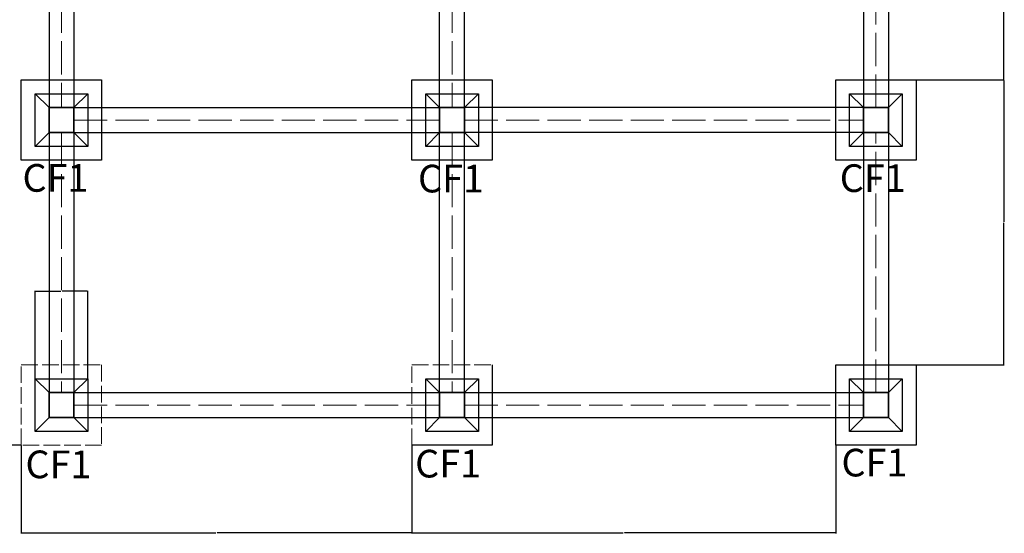
# Model space of a CAD drawing. Units: inches. Extents: x -154 to 668, y -797 to 97.
# Tile 2 of 4: x 313 to 668, y -552 to -367. Entities that reach past the tile are written whole.
import ezdxf

# ---------------------------------------------------------------- set-up
doc = ezdxf.new("R2010")
doc.units = ezdxf.units.IN
doc.header["$MEASUREMENT"] = 0
doc.linetypes.add('ACAD_ISO02W100', pattern=[15, 12, -3])
for name, color, linetype, lineweight in [('A-ANNO-DIMS', 2, 'Continuous', 18), ('S-ANNO-IDEN', 7, 'Continuous', 18), ('S-BEAM', 152, 'Continuous', 25), ('S-BEAM-CNTR', 2, 'ACAD_ISO02W100', 13), ('S-COLS', 2, 'Continuous', 35), ('S-FNDN', 2, 'Continuous', 30), ('S-FNDN-BASE-HIDN', 7, 'ACAD_ISO02W100', 18)]:
    doc.layers.add(name, color=color, linetype=linetype, lineweight=lineweight)
doc.styles.get("Standard").update_dxf_attribs({"font": 'arial.ttf'})
doc.dimstyles.get("Standard").update_dxf_attribs({"dimtxt": 0.18, "dimasz": 0.18, "dimexe": 0.18, "dimexo": 0.0625, "dimgap": 0.09, "dimtad": 0, "dimtih": 1, "dimtoh": 1, "dimdec": 1, "dimzin": 0, "dimdsep": 46, "dimlunit": 4, "dimtxsty": 'Standard', "dimcen": 0.09, "dimadec": 0, "dimazin": 0, "dimtfac": 1, "dimtdec": 1, "dimtofl": 0, "dimtmove": 0, "dimatfit": 3, "dimfxl": 1, "dimtolj": 1, "dimtzin": 0, "dimarcsym": 0})

# ---------------------------------------------------------------- blocks, each defined once
blk = doc.blocks.new('COLUMN-9X9')
for p, q in [((-4.5, 4.5), (4.5, 4.5)), ((-4.5, -4.5), (-4.5, 4.5)), ((4.5, 4.5), (4.5, -4.5)), ((4.5, -4.5), (-4.5, -4.5))]:
    blk.add_line(p, q)
blk = doc.blocks.new('CF1-ISOLATED-FOOTING')
for p, q in [((-14.5, 14.5), (14.5, 14.5)), ((-14.5, -14.5), (-14.5, 14.5)), ((14.5, 14.5), (14.5, -14.5)), ((-9.5, 9.5), (9.5, 9.5)), ((-9.5, -9.5), (-9.5, 9.5)), ((-9.5, 9.5), (-4.5, 4.5)), ((4.5, 4.5), (9.5, 9.5)), ((9.5, 9.5), (9.5, -9.5)), ((-9.5, -9.5), (-4.5, -4.5)), ((4.5, -4.5), (9.5, -9.5)), ((9.5, -9.5), (-9.5, -9.5)), ((14.5, -14.5), (-14.5, -14.5))]:
    blk.add_line(p, q)
blk = doc.blocks.new('*D51')
at = {"layer": 'A-ANNO-DIMS', "color": 0, "lineweight": -2, "transparency": 16777216}
for p, q in [((313.34, 65.33), (281.57, 65.33)), ((281.75, 65.15), (281.75, -227.49)), ((281.75, -520.49), (281.75, -227.85)), ((313.34, -520.67), (281.57, -520.67))]:
    blk.add_line(p, q, dxfattribs=at)
at = {"layer": 'A-ANNO-DIMS', "color": 0, "transparency": 16777216}
for points in [[(281.72, 65.15), (281.78, 65.15), (281.75, 65.33)], [(281.72, -520.49), (281.78, -520.49), (281.75, -520.67)]]:
    blk.add_solid(points, dxfattribs=at)
at = {"layer": 'Defpoints', "color": 0, "transparency": 16777216}
for p in [(281.75, 65.33), (313.4, 65.33), (313.4, -520.67)]:
    blk.add_point(p, dxfattribs=at)
at = {"layer": 'A-ANNO-DIMS', "color": 0, "transparency": 16777216, "insert": (281.75, -227.67), "char_height": 0.18, "attachment_point": 5}
blk.add_mtext('\\A1;586', dxfattribs=at)
blk = doc.blocks.new('*D52')
at = {"layer": 'A-ANNO-DIMS', "color": 0, "lineweight": -2, "transparency": 16777216}
for p, q in [((313.4, -520.73), (313.4, -552.5)), ((454.4, -520.73), (454.4, -552.5)), ((313.58, -552.32), (383.64, -552.32)), ((454.22, -552.32), (384.16, -552.32))]:
    blk.add_line(p, q, dxfattribs=at)
at = {"layer": 'A-ANNO-DIMS', "color": 0, "transparency": 16777216}
for points in [[(313.58, -552.29), (313.58, -552.35), (313.4, -552.32)], [(454.22, -552.29), (454.22, -552.35), (454.4, -552.32)]]:
    blk.add_solid(points, dxfattribs=at)
at = {"layer": 'Defpoints', "color": 0, "transparency": 16777216}
for p in [(313.4, -520.67), (454.4, -520.67), (454.4, -552.32)]:
    blk.add_point(p, dxfattribs=at)
at = {"layer": 'A-ANNO-DIMS', "color": 0, "transparency": 16777216, "insert": (383.9, -552.32), "char_height": 0.18, "attachment_point": 5}
blk.add_mtext('\\A1;141', dxfattribs=at)
blk = doc.blocks.new('*D53')
at = {"layer": 'A-ANNO-DIMS', "color": 0, "lineweight": -2, "transparency": 16777216}
for p, q in [((454.4, -520.73), (454.4, -552.5)), ((607.4, -520.73), (607.4, -552.5)), ((454.58, -552.32), (530.62, -552.32)), ((607.22, -552.32), (531.18, -552.32))]:
    blk.add_line(p, q, dxfattribs=at)
at = {"layer": 'A-ANNO-DIMS', "color": 0, "transparency": 16777216}
for points in [[(454.58, -552.29), (454.58, -552.35), (454.4, -552.32)], [(607.22, -552.29), (607.22, -552.35), (607.4, -552.32)]]:
    blk.add_solid(points, dxfattribs=at)
at = {"layer": 'Defpoints', "color": 0, "transparency": 16777216}
for p in [(454.4, -520.67), (607.4, -520.67), (607.4, -552.32)]:
    blk.add_point(p, dxfattribs=at)
at = {"layer": 'A-ANNO-DIMS', "color": 0, "transparency": 16777216, "insert": (530.9, -552.32), "char_height": 0.18, "attachment_point": 5}
blk.add_mtext('\\A1;153', dxfattribs=at)
blk = doc.blocks.new('*D59')
at = {"layer": 'A-ANNO-DIMS', "color": 0, "lineweight": -2, "transparency": 16777216}
for p, q in [((636.46, -235.67), (668.23, -235.67)), ((668.05, -235.85), (668.05, -311.99)), ((668.05, -388.49), (668.05, -312.35)), ((636.46, -388.67), (668.23, -388.67))]:
    blk.add_line(p, q, dxfattribs=at)
at = {"layer": 'A-ANNO-DIMS', "color": 0, "transparency": 16777216}
for points in [[(668.02, -235.85), (668.08, -235.85), (668.05, -235.67)], [(668.02, -388.49), (668.08, -388.49), (668.05, -388.67)]]:
    blk.add_solid(points, dxfattribs=at)
at = {"layer": 'Defpoints', "color": 0, "transparency": 16777216}
for p in [(636.4, -235.67), (668.05, -235.67), (636.4, -388.67)]:
    blk.add_point(p, dxfattribs=at)
at = {"layer": 'A-ANNO-DIMS', "color": 0, "transparency": 16777216, "insert": (668.05, -312.17), "char_height": 0.18, "attachment_point": 5}
blk.add_mtext('\\A1;153', dxfattribs=at)
blk = doc.blocks.new('*D60')
at = {"layer": 'A-ANNO-DIMS', "color": 0, "lineweight": -2, "transparency": 16777216}
for p, q in [((636.46, -388.67), (668.23, -388.67)), ((668.05, -388.85), (668.05, -439.99)), ((668.05, -491.49), (668.05, -440.35)), ((636.46, -491.67), (668.23, -491.67))]:
    blk.add_line(p, q, dxfattribs=at)
at = {"layer": 'A-ANNO-DIMS', "color": 0, "transparency": 16777216}
for points in [[(668.02, -388.85), (668.08, -388.85), (668.05, -388.67)], [(668.02, -491.49), (668.08, -491.49), (668.05, -491.67)]]:
    blk.add_solid(points, dxfattribs=at)
at = {"layer": 'Defpoints', "color": 0, "transparency": 16777216}
for p in [(636.4, -388.67), (668.05, -388.67), (636.4, -491.67)]:
    blk.add_point(p, dxfattribs=at)
at = {"layer": 'A-ANNO-DIMS', "color": 0, "transparency": 16777216, "insert": (668.05, -440.17), "char_height": 0.18, "attachment_point": 5}
blk.add_mtext('\\A1;103', dxfattribs=at)
blk = doc.blocks.new('*D61')
at = {"layer": 'A-ANNO-DIMS', "color": 0, "lineweight": -2, "transparency": 16777216}
for p, q in [((318.4, -496.6), (318.4, -464.84)), ((318.58, -465.02), (327.69, -465.02)), ((337.22, -465.02), (328.11, -465.02)), ((337.4, -496.6), (337.4, -464.84))]:
    blk.add_line(p, q, dxfattribs=at)
at = {"layer": 'A-ANNO-DIMS', "color": 0, "transparency": 16777216}
for points in [[(318.58, -464.99), (318.58, -465.05), (318.4, -465.02)], [(337.22, -464.99), (337.22, -465.05), (337.4, -465.02)]]:
    blk.add_solid(points, dxfattribs=at)
at = {"layer": 'Defpoints', "color": 0, "transparency": 16777216}
for p in [(337.4, -465.02), (318.4, -496.67), (337.4, -496.67)]:
    blk.add_point(p, dxfattribs=at)
at = {"layer": 'A-ANNO-DIMS', "color": 0, "transparency": 16777216, "insert": (327.9, -465.02), "char_height": 0.18, "attachment_point": 5}
blk.add_mtext('\\A1;19', dxfattribs=at)

msp = doc.modelspace()

# ---------------------------------------------------------------- linework, layer by layer
at = {"layer": 'S-BEAM'}
for p, q in [((323.3997, -254.6672), (323.3997, -407.6672)), ((332.3997, -254.6672), (332.3997, -398.6672)), ((464.3997, -398.6672), (464.3997, -254.6672)), ((473.3997, -398.6672), (473.3997, -254.6672)), ((617.3997, -254.6672), (617.3997, -398.6672)), ((626.3997, -254.6672), (626.3997, -510.6672)), ((332.3997, -398.6672), (464.3997, -398.6672)), ((617.3997, -398.6672), (473.3997, -398.6672)), ((323.3997, -407.6672), (464.3997, -407.6672)), ((323.3997, -407.6672), (323.3997, -510.6672)), ((332.3997, -407.6672), (332.3997, -501.6672)), ((617.3997, -407.6672), (464.3997, -407.6672)), ((464.3997, -501.6672), (464.3997, -407.6672)), ((473.3997, -501.6672), (473.3997, -407.6672)), ((617.3997, -407.6672), (617.3997, -501.6672)), ((332.3997, -501.6672), (464.3997, -501.6672)), ((464.3997, -501.6672), (617.3997, -501.6672)), ((464.3997, -501.6672), (464.3997, -510.6672)), ((323.3997, -510.6672), (626.3997, -510.6672))]:
    msp.add_line(p, q, dxfattribs=at)
at = {"layer": 'S-BEAM-CNTR'}
for p, q in [((327.8997, -254.6672), (327.8997, -398.6672)), ((468.8997, -254.6672), (468.8997, -398.6672)), ((621.8997, -398.6672), (621.8997, -254.6672)), ((332.3997, -403.1672), (464.3997, -403.1672)), ((473.3997, -403.1672), (617.3997, -403.1672)), ((327.8997, -407.6672), (327.8997, -501.6672)), ((468.8997, -407.6672), (468.8997, -501.6672)), ((621.8997, -501.6672), (621.8997, -407.6672)), ((332.3997, -506.1672), (464.3997, -506.1672)), ((473.3997, -506.1672), (617.3997, -506.1672))]:
    msp.add_line(p, q, dxfattribs=at)
at = {"layer": 'S-COLS'}
msp.add_line((617.3997, -407.6672), (617.3997, -398.6672), dxfattribs=at)
at = {"layer": 'S-FNDN'}
for p, q in [((483.3997, -491.6672), (483.3997, -520.6672)), ((318.3997, -515.6672), (318.3997, -496.6672)), ((318.3997, -496.6672), (337.3997, -496.6672)), ((318.3997, -496.6672), (323.3997, -501.6672)), ((332.3997, -501.6672), (337.3997, -496.6672)), ((337.3997, -496.6672), (337.3997, -515.6672)), ((459.3997, -515.6672), (459.3997, -496.6672)), ((459.3997, -496.6672), (478.3997, -496.6672)), ((459.3997, -496.6672), (464.3997, -501.6672)), ((473.3997, -501.6672), (478.3997, -496.6672)), ((478.3997, -496.6672), (478.3997, -515.6672)), ((318.3997, -515.6672), (323.3997, -510.6672)), ((332.3997, -510.6672), (337.3997, -515.6672)), ((459.3997, -515.6672), (464.3997, -510.6672)), ((473.3997, -510.6672), (478.3997, -515.6672)), ((337.3997, -515.6672), (318.3997, -515.6672)), ((478.3997, -515.6672), (459.3997, -515.6672)), ((483.3997, -520.6672), (454.3997, -520.6672))]:
    msp.add_line(p, q, dxfattribs=at)
at = {"layer": 'S-FNDN-BASE-HIDN', "ltscale": 0.5}
for p, q in [((313.3997, -520.6672), (313.3997, -491.6672)), ((313.3997, -491.6672), (342.3997, -491.6672)), ((342.3997, -491.6672), (342.3997, -520.6672)), ((454.3997, -520.6672), (454.3997, -491.6672)), ((454.3997, -491.6672), (483.3997, -491.6672)), ((342.3997, -520.6672), (313.3997, -520.6672))]:
    msp.add_line(p, q, dxfattribs=at)

# ---------------------------------------------------------------- block references
at = {"layer": 'S-COLS'}
for p, rotation in [((327.8995, -403.1669), 89.99999999999893), ((468.8995, -403.1669), 90.00000000000036), ((621.8995, -403.1669), 89.99999999999964), ((327.8995, -506.1669), 89.99999999999893), ((468.8995, -506.1669), 90.00000000000074), ((621.8995, -506.1669), 89.99999999999964)]:
    msp.add_blockref('COLUMN-9X9', p, dxfattribs=dict(at, rotation=rotation))
at = {"layer": 'S-FNDN'}
msp.add_blockref('CF1-ISOLATED-FOOTING', (327.9, -403.167), dxfattribs=at)
for p, rotation in [((468.8994, -403.1674), 180), ((621.8994, -403.1674), 180), ((621.8995, -506.1669), 90.00000000000094)]:
    msp.add_blockref('CF1-ISOLATED-FOOTING', p, dxfattribs=dict(at, rotation=rotation))

# ---------------------------------------------------------------- texts
at = {"layer": 'S-ANNO-IDEN'}
for p in [(313.8292, -429.0678), (456.6003, -429.324), (608.8568, -429.1612), (314.9035, -532.5782), (455.5679, -532.3219), (609.4674, -531.9476)]:
    msp.add_text('CF1', height=10, dxfattribs=at).set_placement(p)

# ---------------------------------------------------------------- dimensions: what is measured, and where the dimension line sits
at = {"layer": 'A-ANNO-DIMS'}
for base, p1, p2, picture, middle in [((281.7497, 65.3328), (313.3997, -520.6672), (313.3997, 65.3328), '*D51', (281.7497, -227.6672)), ((668.0497, -235.6672), (636.3997, -388.6672), (636.3997, -235.6672), '*D59', (668.0497, -312.1672)), ((668.0497, -388.6672), (636.3997, -491.6672), (636.3997, -388.6672), '*D60', (668.0497, -440.1672))]:
    dim = msp.add_linear_dim(base=base, p1=p1, p2=p2, angle=90, dimstyle='Standard', override={"dimdec": 0, "dimlfac": 1, "dimrnd": 0, "dimzin": 0, "dimdsep": 46, "dimlunit": 2}, dxfattribs=at)
    dim.commit()
    dim.dimension.update_dxf_attribs({"geometry": picture, "text_midpoint": middle})
for base, p1, p2, picture, middle in [((337.3997, -465.0172), (318.3997, -496.6672), (337.3997, -496.6672), '*D61', (327.8997, -465.0172)), ((454.3997, -552.3172), (313.3997, -520.6672), (454.3997, -520.6672), '*D52', (383.8997, -552.3172)), ((607.3997, -552.3172), (454.3997, -520.6672), (607.3997, -520.6672), '*D53', (530.8997, -552.3172))]:
    dim = msp.add_linear_dim(base=base, p1=p1, p2=p2, dimstyle='Standard', override={"dimdec": 0, "dimlfac": 1, "dimrnd": 0, "dimzin": 0, "dimdsep": 46, "dimlunit": 2}, dxfattribs=at)
    dim.commit()
    dim.dimension.update_dxf_attribs({"geometry": picture, "text_midpoint": middle})

doc.saveas('drawing.dxf')
